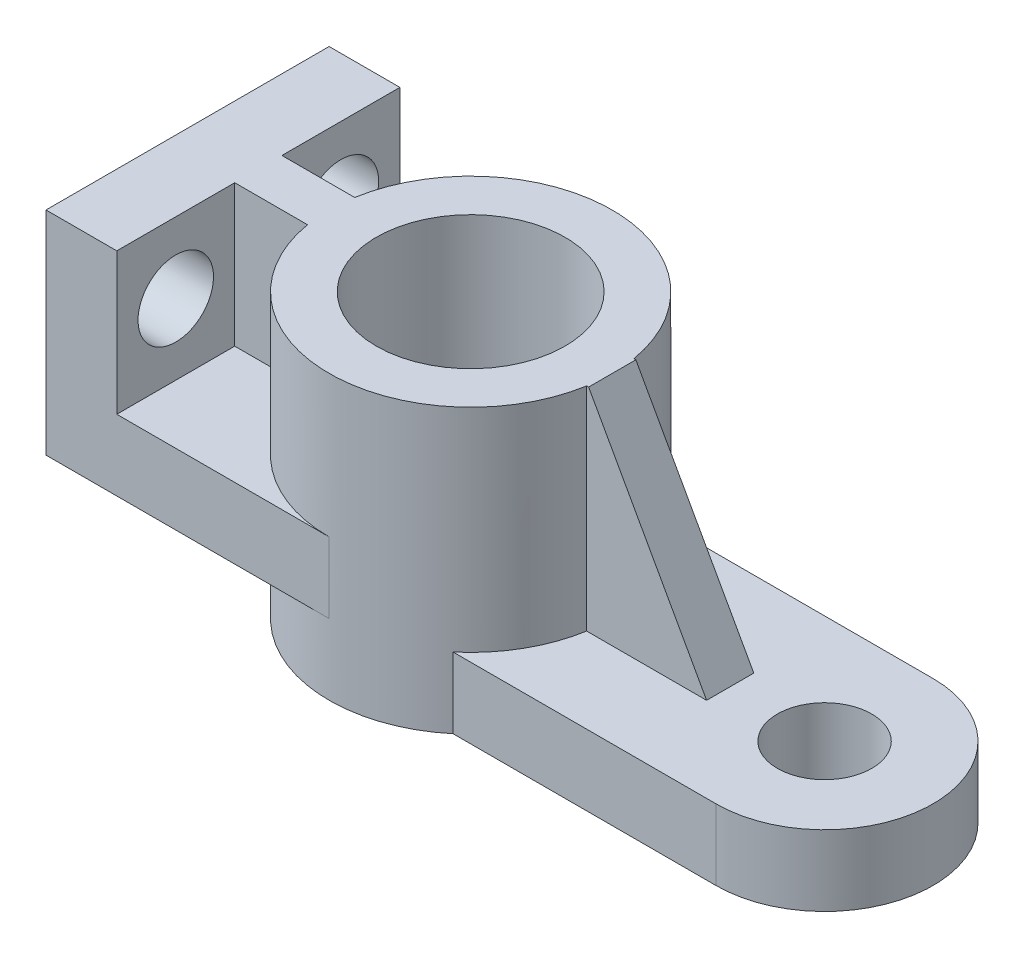
ISO-10303-21;
HEADER;
FILE_DESCRIPTION(('STEP AP214'),'2;1');
FILE_NAME('part.step','',(''),(''),'','','');
FILE_SCHEMA(('AUTOMOTIVE_DESIGN { 1 0 10303 214 1 1 1 1 }'));
ENDSEC;
DATA;
#1=APPLICATION_CONTEXT('core data for automotive mechanical design processes');
#2=APPLICATION_PROTOCOL_DEFINITION('international standard','automotive_design',2000,#1);
#3=PRODUCT_CONTEXT('',#1,'mechanical');
#4=PRODUCT('Part','Part','',(#3));
#5=PRODUCT_RELATED_PRODUCT_CATEGORY('part','',(#4));
#6=PRODUCT_DEFINITION_FORMATION('','',#4);
#7=PRODUCT_DEFINITION_CONTEXT('part definition',#1,'design');
#8=PRODUCT_DEFINITION('design','',#6,#7);
#9=PRODUCT_DEFINITION_SHAPE('','',#8);
#10=(LENGTH_UNIT() NAMED_UNIT(*) SI_UNIT(.MILLI.,.METRE.));
#11=(NAMED_UNIT(*) PLANE_ANGLE_UNIT() SI_UNIT($,.RADIAN.));
#12=(NAMED_UNIT(*) SI_UNIT($,.STERADIAN.) SOLID_ANGLE_UNIT());
#13=UNCERTAINTY_MEASURE_WITH_UNIT(LENGTH_MEASURE(1.E-05),#10,'distance_accuracy_value','');
#14=(GEOMETRIC_REPRESENTATION_CONTEXT(3) GLOBAL_UNCERTAINTY_ASSIGNED_CONTEXT((#13)) GLOBAL_UNIT_ASSIGNED_CONTEXT((#10,
#11,#12)) REPRESENTATION_CONTEXT('',''));
#15=CARTESIAN_POINT('',(0.,0.,0.));
#16=DIRECTION('',(0.,0.,1.));
#17=DIRECTION('',(1.,0.,0.));
#18=AXIS2_PLACEMENT_3D('',#15,#16,#17);
#19=CARTESIAN_POINT('',(0.,60.,0.));
#20=DIRECTION('',(0.,-1.,0.));
#21=DIRECTION('',(0.,0.,-1.));
#22=AXIS2_PLACEMENT_3D('',#19,#20,#21);
#23=CYLINDRICAL_SURFACE('',#22,30.);
#24=CARTESIAN_POINT('',(0.,15.,0.));
#25=DIRECTION('',(0.,-1.,0.));
#26=DIRECTION('',(0.,0.,-1.));
#27=AXIS2_PLACEMENT_3D('',#24,#25,#26);
#28=CIRCLE('',#27,30.);
#29=CARTESIAN_POINT('',(29.5803989154981,15.,5.));
#30=VERTEX_POINT('',#29);
#31=CARTESIAN_POINT('',(19.2613602842582,15.,23.));
#32=VERTEX_POINT('',#31);
#33=EDGE_CURVE('E251',#30,#32,#28,.T.);
#34=ORIENTED_EDGE('',*,*,#33,.F.);
#35=DIRECTION('',(0.,-1.,0.));
#36=VECTOR('',#35,1.);
#37=CARTESIAN_POINT('',(29.5803989154981,60.,5.));
#38=LINE('',#37,#36);
#39=CARTESIAN_POINT('',(29.5803989154981,60.,5.));
#40=VERTEX_POINT('',#39);
#41=EDGE_CURVE('E64',#30,#40,#38,.F.);
#42=ORIENTED_EDGE('',*,*,#41,.T.);
#43=CARTESIAN_POINT('',(0.,60.,0.));
#44=DIRECTION('',(0.,1.,0.));
#45=DIRECTION('',(0.,0.,1.));
#46=AXIS2_PLACEMENT_3D('',#43,#44,#45);
#47=CIRCLE('',#46,30.);
#48=CARTESIAN_POINT('',(-29.5803989154981,60.,5.));
#49=VERTEX_POINT('',#48);
#50=EDGE_CURVE('E189',#49,#40,#47,.T.);
#51=ORIENTED_EDGE('',*,*,#50,.F.);
#52=DIRECTION('',(0.,-1.,0.));
#53=VECTOR('',#52,1.);
#54=CARTESIAN_POINT('',(-29.5803989154981,60.,5.));
#55=LINE('',#54,#53);
#56=CARTESIAN_POINT('',(-29.5803989154981,30.,5.));
#57=VERTEX_POINT('',#56);
#58=EDGE_CURVE('E211',#57,#49,#55,.F.);
#59=ORIENTED_EDGE('',*,*,#58,.F.);
#60=CARTESIAN_POINT('',(0.,30.,0.));
#61=DIRECTION('',(0.,1.,0.));
#62=DIRECTION('',(0.,0.,1.));
#63=AXIS2_PLACEMENT_3D('',#60,#61,#62);
#64=CIRCLE('',#63,30.);
#65=CARTESIAN_POINT('',(0.,30.,30.));
#66=VERTEX_POINT('',#65);
#67=EDGE_CURVE('E268',#66,#57,#64,.F.);
#68=ORIENTED_EDGE('',*,*,#67,.F.);
#69=DIRECTION('',(0.,-1.,0.));
#70=VECTOR('',#69,1.);
#71=CARTESIAN_POINT('',(0.,0.,30.));
#72=LINE('',#71,#70);
#73=CARTESIAN_POINT('',(0.,15.,30.));
#74=VERTEX_POINT('',#73);
#75=EDGE_CURVE('E282',#66,#74,#72,.T.);
#76=ORIENTED_EDGE('',*,*,#75,.T.);
#77=CARTESIAN_POINT('',(0.,15.,0.));
#78=DIRECTION('',(0.,1.,0.));
#79=DIRECTION('',(-1.,0.,0.));
#80=AXIS2_PLACEMENT_3D('',#77,#78,#79);
#81=CIRCLE('',#80,30.);
#82=CARTESIAN_POINT('',(0.,15.,-30.));
#83=VERTEX_POINT('',#82);
#84=EDGE_CURVE('E275',#74,#83,#81,.F.);
#85=ORIENTED_EDGE('',*,*,#84,.T.);
#86=DIRECTION('',(0.,-1.,0.));
#87=VECTOR('',#86,1.);
#88=CARTESIAN_POINT('',(0.,0.,-30.));
#89=LINE('',#88,#87);
#90=CARTESIAN_POINT('',(0.,30.,-30.));
#91=VERTEX_POINT('',#90);
#92=EDGE_CURVE('E299',#91,#83,#89,.T.);
#93=ORIENTED_EDGE('',*,*,#92,.F.);
#94=CARTESIAN_POINT('',(-29.5803989154981,30.,-5.));
#95=VERTEX_POINT('',#94);
#96=EDGE_CURVE('E270',#95,#91,#64,.F.);
#97=ORIENTED_EDGE('',*,*,#96,.F.);
#98=DIRECTION('',(0.,-1.,0.));
#99=VECTOR('',#98,1.);
#100=CARTESIAN_POINT('',(-29.5803989154981,60.,-5.));
#101=LINE('',#100,#99);
#102=CARTESIAN_POINT('',(-29.5803989154981,60.,-5.));
#103=VERTEX_POINT('',#102);
#104=EDGE_CURVE('E215',#103,#95,#101,.T.);
#105=ORIENTED_EDGE('',*,*,#104,.F.);
#106=CARTESIAN_POINT('',(29.5803989154981,60.,-5.));
#107=VERTEX_POINT('',#106);
#108=EDGE_CURVE('E57',#107,#103,#47,.T.);
#109=ORIENTED_EDGE('',*,*,#108,.F.);
#110=DIRECTION('',(0.,-1.,0.));
#111=VECTOR('',#110,1.);
#112=CARTESIAN_POINT('',(29.5803989154981,60.,-5.));
#113=LINE('',#112,#111);
#114=CARTESIAN_POINT('',(29.5803989154981,15.,-5.));
#115=VERTEX_POINT('',#114);
#116=EDGE_CURVE('E193',#115,#107,#113,.F.);
#117=ORIENTED_EDGE('',*,*,#116,.F.);
#118=CARTESIAN_POINT('',(19.2613602842582,15.,-23.));
#119=VERTEX_POINT('',#118);
#120=EDGE_CURVE('E260',#119,#115,#28,.T.);
#121=ORIENTED_EDGE('',*,*,#120,.F.);
#122=DIRECTION('',(0.,1.,0.));
#123=VECTOR('',#122,1.);
#124=CARTESIAN_POINT('',(19.2613602842582,0.,-23.));
#125=LINE('',#124,#123);
#126=CARTESIAN_POINT('',(19.2613602842582,0.,-23.));
#127=VERTEX_POINT('',#126);
#128=EDGE_CURVE('E235',#127,#119,#125,.T.);
#129=ORIENTED_EDGE('',*,*,#128,.F.);
#130=CARTESIAN_POINT('',(0.,0.,0.));
#131=DIRECTION('',(0.,1.,0.));
#132=DIRECTION('',(0.,0.,1.));
#133=AXIS2_PLACEMENT_3D('',#130,#131,#132);
#134=CIRCLE('',#133,30.);
#135=CARTESIAN_POINT('',(19.2613602842582,0.,23.));
#136=VERTEX_POINT('',#135);
#137=EDGE_CURVE('E264',#127,#136,#134,.T.);
#138=ORIENTED_EDGE('',*,*,#137,.T.);
#139=DIRECTION('',(0.,1.,0.));
#140=VECTOR('',#139,1.);
#141=CARTESIAN_POINT('',(19.2613602842582,0.,23.));
#142=LINE('',#141,#140);
#143=EDGE_CURVE('E232',#136,#32,#142,.T.);
#144=ORIENTED_EDGE('',*,*,#143,.T.);
#145=EDGE_LOOP('',(#34,#42,#51,#59,#68,#76,#85,#93,#97,#105,#109,#117,#121,#129,#138,#144));
#146=FACE_BOUND('',#145,.T.);
#147=ADVANCED_FACE('F41',(#146),#23,.T.);
#148=CARTESIAN_POINT('',(0.,30.,30.));
#149=DIRECTION('',(0.,1.,0.));
#150=DIRECTION('',(0.,0.,1.));
#151=AXIS2_PLACEMENT_3D('',#148,#149,#150);
#152=PLANE('',#151);
#153=ORIENTED_EDGE('',*,*,#67,.T.);
#154=DIRECTION('',(-1.,0.,0.));
#155=VECTOR('',#154,1.);
#156=CARTESIAN_POINT('',(-27.,30.,5.));
#157=LINE('',#156,#155);
#158=CARTESIAN_POINT('',(-45.,30.,5.));
#159=VERTEX_POINT('',#158);
#160=EDGE_CURVE('E210',#57,#159,#157,.T.);
#161=ORIENTED_EDGE('',*,*,#160,.T.);
#162=DIRECTION('',(0.,0.,-1.));
#163=VECTOR('',#162,1.);
#164=CARTESIAN_POINT('',(-45.,30.,30.));
#165=LINE('',#164,#163);
#166=CARTESIAN_POINT('',(-45.,30.,30.));
#167=VERTEX_POINT('',#166);
#168=EDGE_CURVE('E317',#167,#159,#165,.T.);
#169=ORIENTED_EDGE('',*,*,#168,.F.);
#170=DIRECTION('',(1.,0.,0.));
#171=VECTOR('',#170,1.);
#172=CARTESIAN_POINT('',(0.,30.,30.));
#173=LINE('',#172,#171);
#174=EDGE_CURVE('E283',#167,#66,#173,.T.);
#175=ORIENTED_EDGE('',*,*,#174,.T.);
#176=EDGE_LOOP('',(#153,#161,#169,#175));
#177=FACE_BOUND('',#176,.T.);
#178=ADVANCED_FACE('F334',(#177),#152,.T.);
#179=CARTESIAN_POINT('',(-45.,30.,-5.));
#180=VERTEX_POINT('',#179);
#181=CARTESIAN_POINT('',(-45.,30.,-30.));
#182=VERTEX_POINT('',#181);
#183=EDGE_CURVE('E314',#180,#182,#165,.T.);
#184=ORIENTED_EDGE('',*,*,#183,.F.);
#185=DIRECTION('',(-1.,0.,0.));
#186=VECTOR('',#185,1.);
#187=CARTESIAN_POINT('',(-27.,30.,-5.));
#188=LINE('',#187,#186);
#189=EDGE_CURVE('E204',#95,#180,#188,.T.);
#190=ORIENTED_EDGE('',*,*,#189,.F.);
#191=ORIENTED_EDGE('',*,*,#96,.T.);
#192=DIRECTION('',(1.,0.,0.));
#193=VECTOR('',#192,1.);
#194=CARTESIAN_POINT('',(0.,30.,-30.));
#195=LINE('',#194,#193);
#196=EDGE_CURVE('E305',#182,#91,#195,.T.);
#197=ORIENTED_EDGE('',*,*,#196,.F.);
#198=EDGE_LOOP('',(#184,#190,#191,#197));
#199=FACE_BOUND('',#198,.T.);
#200=ADVANCED_FACE('F345',(#199),#152,.T.);
#201=CARTESIAN_POINT('',(-45.,0.,30.));
#202=DIRECTION('',(1.,0.,0.));
#203=DIRECTION('',(0.,1.,0.));
#204=AXIS2_PLACEMENT_3D('',#201,#202,#203);
#205=PLANE('',#204);
#206=CARTESIAN_POINT('',(-45.,45.,17.5));
#207=DIRECTION('',(1.,0.,0.));
#208=DIRECTION('',(0.,1.,0.));
#209=AXIS2_PLACEMENT_3D('',#206,#207,#208);
#210=CIRCLE('',#209,8.);
#211=CARTESIAN_POINT('',(-45.,53.,17.5));
#212=VERTEX_POINT('',#211);
#213=EDGE_CURVE('E221',#212,#212,#210,.T.);
#214=ORIENTED_EDGE('',*,*,#213,.F.);
#215=EDGE_LOOP('',(#214));
#216=FACE_BOUND('',#215,.T.);
#217=ORIENTED_EDGE('',*,*,#168,.T.);
#218=DIRECTION('',(0.,-1.,0.));
#219=VECTOR('',#218,1.);
#220=CARTESIAN_POINT('',(-45.,30.,5.));
#221=LINE('',#220,#219);
#222=CARTESIAN_POINT('',(-45.,60.,5.));
#223=VERTEX_POINT('',#222);
#224=EDGE_CURVE('E199',#223,#159,#221,.T.);
#225=ORIENTED_EDGE('',*,*,#224,.F.);
#226=DIRECTION('',(0.,0.,-1.));
#227=VECTOR('',#226,1.);
#228=CARTESIAN_POINT('',(-45.,60.,30.));
#229=LINE('',#228,#227);
#230=CARTESIAN_POINT('',(-45.,60.,30.));
#231=VERTEX_POINT('',#230);
#232=EDGE_CURVE('E315',#231,#223,#229,.T.);
#233=ORIENTED_EDGE('',*,*,#232,.F.);
#234=DIRECTION('',(0.,-1.,0.));
#235=VECTOR('',#234,1.);
#236=CARTESIAN_POINT('',(-45.,0.,30.));
#237=LINE('',#236,#235);
#238=EDGE_CURVE('E290',#231,#167,#237,.T.);
#239=ORIENTED_EDGE('',*,*,#238,.T.);
#240=EDGE_LOOP('',(#217,#225,#233,#239));
#241=FACE_BOUND('',#240,.T.);
#242=ADVANCED_FACE('F361',(#216,#241),#205,.T.);
#243=CARTESIAN_POINT('',(-45.,45.,-17.5));
#244=DIRECTION('',(1.,0.,0.));
#245=DIRECTION('',(0.,-1.,0.));
#246=AXIS2_PLACEMENT_3D('',#243,#244,#245);
#247=CIRCLE('',#246,8.);
#248=CARTESIAN_POINT('',(-45.,37.,-17.5));
#249=VERTEX_POINT('',#248);
#250=EDGE_CURVE('E216',#249,#249,#247,.T.);
#251=ORIENTED_EDGE('',*,*,#250,.F.);
#252=EDGE_LOOP('',(#251));
#253=FACE_BOUND('',#252,.T.);
#254=CARTESIAN_POINT('',(-45.,60.,-5.));
#255=VERTEX_POINT('',#254);
#256=CARTESIAN_POINT('',(-45.,60.,-30.));
#257=VERTEX_POINT('',#256);
#258=EDGE_CURVE('E311',#255,#257,#229,.T.);
#259=ORIENTED_EDGE('',*,*,#258,.F.);
#260=DIRECTION('',(0.,1.,0.));
#261=VECTOR('',#260,1.);
#262=CARTESIAN_POINT('',(-45.,60.,-5.));
#263=LINE('',#262,#261);
#264=EDGE_CURVE('E200',#180,#255,#263,.T.);
#265=ORIENTED_EDGE('',*,*,#264,.F.);
#266=ORIENTED_EDGE('',*,*,#183,.T.);
#267=DIRECTION('',(0.,-1.,0.));
#268=VECTOR('',#267,1.);
#269=CARTESIAN_POINT('',(-45.,0.,-30.));
#270=LINE('',#269,#268);
#271=EDGE_CURVE('E304',#257,#182,#270,.T.);
#272=ORIENTED_EDGE('',*,*,#271,.F.);
#273=EDGE_LOOP('',(#259,#265,#266,#272));
#274=FACE_BOUND('',#273,.T.);
#275=ADVANCED_FACE('F362',(#253,#274),#205,.T.);
#276=CARTESIAN_POINT('',(0.,15.,30.));
#277=DIRECTION('',(0.,1.,0.));
#278=DIRECTION('',(-1.,0.,0.));
#279=AXIS2_PLACEMENT_3D('',#276,#277,#278);
#280=PLANE('',#279);
#281=ORIENTED_EDGE('',*,*,#84,.F.);
#282=DIRECTION('',(1.,0.,0.));
#283=VECTOR('',#282,1.);
#284=CARTESIAN_POINT('',(0.,15.,30.));
#285=LINE('',#284,#283);
#286=CARTESIAN_POINT('',(-60.,15.,30.));
#287=VERTEX_POINT('',#286);
#288=EDGE_CURVE('E279',#287,#74,#285,.T.);
#289=ORIENTED_EDGE('',*,*,#288,.F.);
#290=DIRECTION('',(0.,0.,-1.));
#291=VECTOR('',#290,1.);
#292=CARTESIAN_POINT('',(-60.,15.,30.));
#293=LINE('',#292,#291);
#294=CARTESIAN_POINT('',(-60.,15.,-30.));
#295=VERTEX_POINT('',#294);
#296=EDGE_CURVE('E316',#287,#295,#293,.T.);
#297=ORIENTED_EDGE('',*,*,#296,.T.);
#298=DIRECTION('',(1.,0.,0.));
#299=VECTOR('',#298,1.);
#300=CARTESIAN_POINT('',(0.,15.,-30.));
#301=LINE('',#300,#299);
#302=EDGE_CURVE('E298',#295,#83,#301,.T.);
#303=ORIENTED_EDGE('',*,*,#302,.T.);
#304=EDGE_LOOP('',(#281,#289,#297,#303));
#305=FACE_BOUND('',#304,.T.);
#306=ADVANCED_FACE('F370',(#305),#280,.F.);
#307=CARTESIAN_POINT('',(-60.,0.,30.));
#308=DIRECTION('',(-1.,0.,0.));
#309=DIRECTION('',(0.,0.,1.));
#310=AXIS2_PLACEMENT_3D('',#307,#308,#309);
#311=PLANE('',#310);
#312=CARTESIAN_POINT('',(-60.,45.,17.5));
#313=DIRECTION('',(1.,0.,0.));
#314=DIRECTION('',(0.,1.,0.));
#315=AXIS2_PLACEMENT_3D('',#312,#313,#314);
#316=CIRCLE('',#315,8.);
#317=CARTESIAN_POINT('',(-60.,53.,17.5));
#318=VERTEX_POINT('',#317);
#319=EDGE_CURVE('E217',#318,#318,#316,.T.);
#320=ORIENTED_EDGE('',*,*,#319,.T.);
#321=EDGE_LOOP('',(#320));
#322=FACE_BOUND('',#321,.T.);
#323=CARTESIAN_POINT('',(-60.,45.,-17.5));
#324=DIRECTION('',(1.,0.,0.));
#325=DIRECTION('',(0.,-1.,0.));
#326=AXIS2_PLACEMENT_3D('',#323,#324,#325);
#327=CIRCLE('',#326,8.);
#328=CARTESIAN_POINT('',(-60.,37.,-17.5));
#329=VERTEX_POINT('',#328);
#330=EDGE_CURVE('E223',#329,#329,#327,.T.);
#331=ORIENTED_EDGE('',*,*,#330,.T.);
#332=EDGE_LOOP('',(#331));
#333=FACE_BOUND('',#332,.T.);
#334=DIRECTION('',(0.,1.,0.));
#335=VECTOR('',#334,1.);
#336=CARTESIAN_POINT('',(-60.,0.,-30.));
#337=LINE('',#336,#335);
#338=CARTESIAN_POINT('',(-60.,60.,-30.));
#339=VERTEX_POINT('',#338);
#340=EDGE_CURVE('E274',#295,#339,#337,.T.);
#341=ORIENTED_EDGE('',*,*,#340,.F.);
#342=ORIENTED_EDGE('',*,*,#296,.F.);
#343=DIRECTION('',(0.,1.,0.));
#344=VECTOR('',#343,1.);
#345=CARTESIAN_POINT('',(-60.,0.,30.));
#346=LINE('',#345,#344);
#347=CARTESIAN_POINT('',(-60.,60.,30.));
#348=VERTEX_POINT('',#347);
#349=EDGE_CURVE('E273',#287,#348,#346,.T.);
#350=ORIENTED_EDGE('',*,*,#349,.T.);
#351=DIRECTION('',(0.,0.,-1.));
#352=VECTOR('',#351,1.);
#353=CARTESIAN_POINT('',(-60.,60.,30.));
#354=LINE('',#353,#352);
#355=EDGE_CURVE('E291',#348,#339,#354,.T.);
#356=ORIENTED_EDGE('',*,*,#355,.T.);
#357=EDGE_LOOP('',(#341,#342,#350,#356));
#358=FACE_BOUND('',#357,.T.);
#359=ADVANCED_FACE('F43',(#322,#333,#358),#311,.T.);
#360=CARTESIAN_POINT('',(0.,60.,30.));
#361=DIRECTION('',(0.,1.,0.));
#362=DIRECTION('',(0.,0.,1.));
#363=AXIS2_PLACEMENT_3D('',#360,#361,#362);
#364=PLANE('',#363);
#365=CARTESIAN_POINT('',(0.,60.,0.));
#366=DIRECTION('',(0.,1.,0.));
#367=DIRECTION('',(0.,0.,1.));
#368=AXIS2_PLACEMENT_3D('',#365,#366,#367);
#369=CIRCLE('',#368,20.);
#370=CARTESIAN_POINT('',(0.,60.,20.));
#371=VERTEX_POINT('',#370);
#372=EDGE_CURVE('E258',#371,#371,#369,.T.);
#373=ORIENTED_EDGE('',*,*,#372,.F.);
#374=EDGE_LOOP('',(#373));
#375=FACE_BOUND('',#374,.T.);
#376=ORIENTED_EDGE('',*,*,#50,.T.);
#377=DIRECTION('',(-1.,0.,0.));
#378=VECTOR('',#377,1.);
#379=CARTESIAN_POINT('',(30.,60.,5.));
#380=LINE('',#379,#378);
#381=CARTESIAN_POINT('',(30.,60.,5.));
#382=VERTEX_POINT('',#381);
#383=EDGE_CURVE('E183',#382,#40,#380,.T.);
#384=ORIENTED_EDGE('',*,*,#383,.F.);
#385=DIRECTION('',(0.,0.,-1.));
#386=VECTOR('',#385,1.);
#387=CARTESIAN_POINT('',(30.,60.,5.));
#388=LINE('',#387,#386);
#389=CARTESIAN_POINT('',(30.,60.,-5.));
#390=VERTEX_POINT('',#389);
#391=EDGE_CURVE('E170',#382,#390,#388,.T.);
#392=ORIENTED_EDGE('',*,*,#391,.T.);
#393=DIRECTION('',(-1.,0.,0.));
#394=VECTOR('',#393,1.);
#395=CARTESIAN_POINT('',(30.,60.,-5.));
#396=LINE('',#395,#394);
#397=EDGE_CURVE('E188',#390,#107,#396,.T.);
#398=ORIENTED_EDGE('',*,*,#397,.T.);
#399=ORIENTED_EDGE('',*,*,#108,.T.);
#400=DIRECTION('',(-1.,0.,0.));
#401=VECTOR('',#400,1.);
#402=CARTESIAN_POINT('',(-27.,60.,-5.));
#403=LINE('',#402,#401);
#404=EDGE_CURVE('E205',#103,#255,#403,.T.);
#405=ORIENTED_EDGE('',*,*,#404,.T.);
#406=ORIENTED_EDGE('',*,*,#258,.T.);
#407=DIRECTION('',(1.,0.,0.));
#408=VECTOR('',#407,1.);
#409=CARTESIAN_POINT('',(0.,60.,-30.));
#410=LINE('',#409,#408);
#411=EDGE_CURVE('E276',#339,#257,#410,.T.);
#412=ORIENTED_EDGE('',*,*,#411,.F.);
#413=ORIENTED_EDGE('',*,*,#355,.F.);
#414=DIRECTION('',(1.,0.,0.));
#415=VECTOR('',#414,1.);
#416=CARTESIAN_POINT('',(0.,60.,30.));
#417=LINE('',#416,#415);
#418=EDGE_CURVE('E289',#348,#231,#417,.T.);
#419=ORIENTED_EDGE('',*,*,#418,.T.);
#420=ORIENTED_EDGE('',*,*,#232,.T.);
#421=DIRECTION('',(-1.,0.,0.));
#422=VECTOR('',#421,1.);
#423=CARTESIAN_POINT('',(-27.,60.,5.));
#424=LINE('',#423,#422);
#425=EDGE_CURVE('E208',#49,#223,#424,.T.);
#426=ORIENTED_EDGE('',*,*,#425,.F.);
#427=EDGE_LOOP('',(#376,#384,#392,#398,#399,#405,#406,#412,#413,#419,#420,#426));
#428=FACE_BOUND('',#427,.T.);
#429=ADVANCED_FACE('F187',(#375,#428),#364,.T.);
#430=CARTESIAN_POINT('',(0.,0.,30.));
#431=DIRECTION('',(0.,0.,1.));
#432=DIRECTION('',(1.,0.,0.));
#433=AXIS2_PLACEMENT_3D('',#430,#431,#432);
#434=PLANE('',#433);
#435=ORIENTED_EDGE('',*,*,#349,.F.);
#436=ORIENTED_EDGE('',*,*,#288,.T.);
#437=ORIENTED_EDGE('',*,*,#75,.F.);
#438=ORIENTED_EDGE('',*,*,#174,.F.);
#439=ORIENTED_EDGE('',*,*,#238,.F.);
#440=ORIENTED_EDGE('',*,*,#418,.F.);
#441=EDGE_LOOP('',(#435,#436,#437,#438,#439,#440));
#442=FACE_BOUND('',#441,.T.);
#443=ADVANCED_FACE('F352',(#442),#434,.T.);
#444=CARTESIAN_POINT('',(0.,0.,-30.));
#445=DIRECTION('',(0.,0.,1.));
#446=DIRECTION('',(1.,0.,0.));
#447=AXIS2_PLACEMENT_3D('',#444,#445,#446);
#448=PLANE('',#447);
#449=ORIENTED_EDGE('',*,*,#340,.T.);
#450=ORIENTED_EDGE('',*,*,#411,.T.);
#451=ORIENTED_EDGE('',*,*,#271,.T.);
#452=ORIENTED_EDGE('',*,*,#196,.T.);
#453=ORIENTED_EDGE('',*,*,#92,.T.);
#454=ORIENTED_EDGE('',*,*,#302,.F.);
#455=EDGE_LOOP('',(#449,#450,#451,#452,#453,#454));
#456=FACE_BOUND('',#455,.T.);
#457=ADVANCED_FACE('F358',(#456),#448,.F.);
#458=CARTESIAN_POINT('',(0.,0.,0.));
#459=DIRECTION('',(0.,1.,0.));
#460=DIRECTION('',(0.,0.,1.));
#461=AXIS2_PLACEMENT_3D('',#458,#459,#460);
#462=PLANE('',#461);
#463=CARTESIAN_POINT('',(75.,0.,0.));
#464=DIRECTION('',(0.,1.,0.));
#465=DIRECTION('',(0.,0.,1.));
#466=AXIS2_PLACEMENT_3D('',#463,#464,#465);
#467=CIRCLE('',#466,9.99999999999999);
#468=CARTESIAN_POINT('',(75.,0.,9.99999999999999));
#469=VERTEX_POINT('',#468);
#470=EDGE_CURVE('E244',#469,#469,#467,.T.);
#471=ORIENTED_EDGE('',*,*,#470,.T.);
#472=EDGE_LOOP('',(#471));
#473=FACE_BOUND('',#472,.T.);
#474=CARTESIAN_POINT('',(75.,0.,0.));
#475=DIRECTION('',(0.,1.,0.));
#476=DIRECTION('',(0.,0.,1.));
#477=AXIS2_PLACEMENT_3D('',#474,#475,#476);
#478=CIRCLE('',#477,23.);
#479=CARTESIAN_POINT('',(75.,0.,23.));
#480=VERTEX_POINT('',#479);
#481=CARTESIAN_POINT('',(75.,0.,-23.));
#482=VERTEX_POINT('',#481);
#483=EDGE_CURVE('E247',#480,#482,#478,.T.);
#484=ORIENTED_EDGE('',*,*,#483,.F.);
#485=DIRECTION('',(-1.,0.,0.));
#486=VECTOR('',#485,1.);
#487=CARTESIAN_POINT('',(74.9999999999999,0.,23.));
#488=LINE('',#487,#486);
#489=EDGE_CURVE('E238',#480,#136,#488,.T.);
#490=ORIENTED_EDGE('',*,*,#489,.T.);
#491=ORIENTED_EDGE('',*,*,#137,.F.);
#492=DIRECTION('',(1.,0.,0.));
#493=VECTOR('',#492,1.);
#494=CARTESIAN_POINT('',(75.,0.,-23.));
#495=LINE('',#494,#493);
#496=EDGE_CURVE('E230',#127,#482,#495,.T.);
#497=ORIENTED_EDGE('',*,*,#496,.T.);
#498=EDGE_LOOP('',(#484,#490,#491,#497));
#499=FACE_BOUND('',#498,.T.);
#500=CARTESIAN_POINT('',(0.,0.,0.));
#501=DIRECTION('',(0.,1.,0.));
#502=DIRECTION('',(0.,0.,1.));
#503=AXIS2_PLACEMENT_3D('',#500,#501,#502);
#504=CIRCLE('',#503,20.);
#505=CARTESIAN_POINT('',(0.,0.,20.));
#506=VERTEX_POINT('',#505);
#507=EDGE_CURVE('E256',#506,#506,#504,.T.);
#508=ORIENTED_EDGE('',*,*,#507,.T.);
#509=EDGE_LOOP('',(#508));
#510=FACE_BOUND('',#509,.T.);
#511=ADVANCED_FACE('F347',(#473,#499,#510),#462,.F.);
#512=CARTESIAN_POINT('',(0.,60.,0.));
#513=DIRECTION('',(0.,-1.,0.));
#514=DIRECTION('',(0.,0.,-1.));
#515=AXIS2_PLACEMENT_3D('',#512,#513,#514);
#516=CYLINDRICAL_SURFACE('',#515,20.);
#517=ORIENTED_EDGE('',*,*,#507,.F.);
#518=EDGE_LOOP('',(#517));
#519=FACE_BOUND('',#518,.T.);
#520=ORIENTED_EDGE('',*,*,#372,.T.);
#521=EDGE_LOOP('',(#520));
#522=FACE_BOUND('',#521,.T.);
#523=ADVANCED_FACE('F348',(#519,#522),#516,.F.);
#524=CARTESIAN_POINT('',(0.,15.,30.));
#525=DIRECTION('',(0.,-1.,0.));
#526=DIRECTION('',(0.,0.,-1.));
#527=AXIS2_PLACEMENT_3D('',#524,#525,#526);
#528=PLANE('',#527);
#529=CARTESIAN_POINT('',(75.,15.,0.));
#530=DIRECTION('',(0.,1.,0.));
#531=DIRECTION('',(0.,0.,1.));
#532=AXIS2_PLACEMENT_3D('',#529,#530,#531);
#533=CIRCLE('',#532,9.99999999999999);
#534=CARTESIAN_POINT('',(75.,15.,9.99999999999999));
#535=VERTEX_POINT('',#534);
#536=EDGE_CURVE('E240',#535,#535,#533,.T.);
#537=ORIENTED_EDGE('',*,*,#536,.F.);
#538=EDGE_LOOP('',(#537));
#539=FACE_BOUND('',#538,.T.);
#540=DIRECTION('',(0.,0.,-1.));
#541=VECTOR('',#540,1.);
#542=CARTESIAN_POINT('',(55.,15.,5.));
#543=LINE('',#542,#541);
#544=CARTESIAN_POINT('',(55.,15.,5.));
#545=VERTEX_POINT('',#544);
#546=CARTESIAN_POINT('',(55.,15.,-5.));
#547=VERTEX_POINT('',#546);
#548=EDGE_CURVE('E178',#545,#547,#543,.T.);
#549=ORIENTED_EDGE('',*,*,#548,.F.);
#550=DIRECTION('',(-1.,0.,0.));
#551=VECTOR('',#550,1.);
#552=CARTESIAN_POINT('',(0.,15.,5.));
#553=LINE('',#552,#551);
#554=EDGE_CURVE('E11',#545,#30,#553,.T.);
#555=ORIENTED_EDGE('',*,*,#554,.T.);
#556=ORIENTED_EDGE('',*,*,#33,.T.);
#557=DIRECTION('',(-1.,0.,0.));
#558=VECTOR('',#557,1.);
#559=CARTESIAN_POINT('',(74.9999999999999,15.,23.));
#560=LINE('',#559,#558);
#561=CARTESIAN_POINT('',(74.9999999999999,15.,23.));
#562=VERTEX_POINT('',#561);
#563=EDGE_CURVE('E220',#562,#32,#560,.T.);
#564=ORIENTED_EDGE('',*,*,#563,.F.);
#565=CARTESIAN_POINT('',(75.,15.,0.));
#566=DIRECTION('',(0.,1.,0.));
#567=DIRECTION('',(0.,0.,1.));
#568=AXIS2_PLACEMENT_3D('',#565,#566,#567);
#569=CIRCLE('',#568,23.);
#570=CARTESIAN_POINT('',(75.,15.,-23.));
#571=VERTEX_POINT('',#570);
#572=EDGE_CURVE('E252',#562,#571,#569,.T.);
#573=ORIENTED_EDGE('',*,*,#572,.T.);
#574=DIRECTION('',(1.,0.,0.));
#575=VECTOR('',#574,1.);
#576=CARTESIAN_POINT('',(75.,15.,-23.));
#577=LINE('',#576,#575);
#578=EDGE_CURVE('E231',#119,#571,#577,.T.);
#579=ORIENTED_EDGE('',*,*,#578,.F.);
#580=ORIENTED_EDGE('',*,*,#120,.T.);
#581=DIRECTION('',(-1.,0.,0.));
#582=VECTOR('',#581,1.);
#583=CARTESIAN_POINT('',(0.,15.,-5.));
#584=LINE('',#583,#582);
#585=EDGE_CURVE('E47',#547,#115,#584,.T.);
#586=ORIENTED_EDGE('',*,*,#585,.F.);
#587=EDGE_LOOP('',(#549,#555,#556,#564,#573,#579,#580,#586));
#588=FACE_BOUND('',#587,.T.);
#589=ADVANCED_FACE('F330',(#539,#588),#528,.F.);
#590=CARTESIAN_POINT('',(75.,15.,0.));
#591=DIRECTION('',(0.,-1.,0.));
#592=DIRECTION('',(0.,0.,-1.));
#593=AXIS2_PLACEMENT_3D('',#590,#591,#592);
#594=CYLINDRICAL_SURFACE('',#593,23.);
#595=ORIENTED_EDGE('',*,*,#483,.T.);
#596=DIRECTION('',(0.,-1.,0.));
#597=VECTOR('',#596,1.);
#598=CARTESIAN_POINT('',(75.,15.,-23.));
#599=LINE('',#598,#597);
#600=EDGE_CURVE('E321',#482,#571,#599,.F.);
#601=ORIENTED_EDGE('',*,*,#600,.T.);
#602=ORIENTED_EDGE('',*,*,#572,.F.);
#603=DIRECTION('',(0.,-1.,0.));
#604=VECTOR('',#603,1.);
#605=CARTESIAN_POINT('',(75.,15.,23.));
#606=LINE('',#605,#604);
#607=EDGE_CURVE('E322',#562,#480,#606,.T.);
#608=ORIENTED_EDGE('',*,*,#607,.T.);
#609=EDGE_LOOP('',(#595,#601,#602,#608));
#610=FACE_BOUND('',#609,.T.);
#611=ADVANCED_FACE('F424',(#610),#594,.T.);
#612=CARTESIAN_POINT('',(75.,0.,-23.));
#613=DIRECTION('',(0.,0.,1.));
#614=DIRECTION('',(1.,0.,0.));
#615=AXIS2_PLACEMENT_3D('',#612,#613,#614);
#616=PLANE('',#615);
#617=ORIENTED_EDGE('',*,*,#578,.T.);
#618=ORIENTED_EDGE('',*,*,#600,.F.);
#619=ORIENTED_EDGE('',*,*,#496,.F.);
#620=ORIENTED_EDGE('',*,*,#128,.T.);
#621=EDGE_LOOP('',(#617,#618,#619,#620));
#622=FACE_BOUND('',#621,.T.);
#623=ADVANCED_FACE('F423',(#622),#616,.F.);
#624=CARTESIAN_POINT('',(74.9999999999999,0.,23.));
#625=DIRECTION('',(0.,0.,-1.));
#626=DIRECTION('',(-1.,0.,0.));
#627=AXIS2_PLACEMENT_3D('',#624,#625,#626);
#628=PLANE('',#627);
#629=ORIENTED_EDGE('',*,*,#563,.T.);
#630=ORIENTED_EDGE('',*,*,#143,.F.);
#631=ORIENTED_EDGE('',*,*,#489,.F.);
#632=ORIENTED_EDGE('',*,*,#607,.F.);
#633=EDGE_LOOP('',(#629,#630,#631,#632));
#634=FACE_BOUND('',#633,.T.);
#635=ADVANCED_FACE('F425',(#634),#628,.F.);
#636=CARTESIAN_POINT('',(75.,0.,0.));
#637=DIRECTION('',(0.,1.,0.));
#638=DIRECTION('',(0.,0.,1.));
#639=AXIS2_PLACEMENT_3D('',#636,#637,#638);
#640=CYLINDRICAL_SURFACE('',#639,9.99999999999999);
#641=ORIENTED_EDGE('',*,*,#470,.F.);
#642=EDGE_LOOP('',(#641));
#643=FACE_BOUND('',#642,.T.);
#644=ORIENTED_EDGE('',*,*,#536,.T.);
#645=EDGE_LOOP('',(#644));
#646=FACE_BOUND('',#645,.T.);
#647=ADVANCED_FACE('F418',(#643,#646),#640,.F.);
#648=CARTESIAN_POINT('',(-60.,45.,-17.5));
#649=DIRECTION('',(1.,0.,0.));
#650=DIRECTION('',(0.,1.,0.));
#651=AXIS2_PLACEMENT_3D('',#648,#649,#650);
#652=CYLINDRICAL_SURFACE('',#651,8.);
#653=ORIENTED_EDGE('',*,*,#330,.F.);
#654=EDGE_LOOP('',(#653));
#655=FACE_BOUND('',#654,.T.);
#656=ORIENTED_EDGE('',*,*,#250,.T.);
#657=EDGE_LOOP('',(#656));
#658=FACE_BOUND('',#657,.T.);
#659=ADVANCED_FACE('F412',(#655,#658),#652,.F.);
#660=CARTESIAN_POINT('',(-60.,45.,17.5));
#661=DIRECTION('',(1.,0.,0.));
#662=DIRECTION('',(0.,1.,0.));
#663=AXIS2_PLACEMENT_3D('',#660,#661,#662);
#664=CYLINDRICAL_SURFACE('',#663,8.);
#665=ORIENTED_EDGE('',*,*,#319,.F.);
#666=EDGE_LOOP('',(#665));
#667=FACE_BOUND('',#666,.T.);
#668=ORIENTED_EDGE('',*,*,#213,.T.);
#669=EDGE_LOOP('',(#668));
#670=FACE_BOUND('',#669,.T.);
#671=ADVANCED_FACE('F407',(#667,#670),#664,.F.);
#672=CARTESIAN_POINT('',(-27.,30.,5.));
#673=DIRECTION('',(0.,0.,-1.));
#674=DIRECTION('',(-1.,0.,0.));
#675=AXIS2_PLACEMENT_3D('',#672,#673,#674);
#676=PLANE('',#675);
#677=ORIENTED_EDGE('',*,*,#160,.F.);
#678=ORIENTED_EDGE('',*,*,#58,.T.);
#679=ORIENTED_EDGE('',*,*,#425,.T.);
#680=ORIENTED_EDGE('',*,*,#224,.T.);
#681=EDGE_LOOP('',(#677,#678,#679,#680));
#682=FACE_BOUND('',#681,.T.);
#683=ADVANCED_FACE('F404',(#682),#676,.F.);
#684=CARTESIAN_POINT('',(-27.,60.,-5.));
#685=DIRECTION('',(0.,0.,1.));
#686=DIRECTION('',(0.,-1.,0.));
#687=AXIS2_PLACEMENT_3D('',#684,#685,#686);
#688=PLANE('',#687);
#689=ORIENTED_EDGE('',*,*,#404,.F.);
#690=ORIENTED_EDGE('',*,*,#104,.T.);
#691=ORIENTED_EDGE('',*,*,#189,.T.);
#692=ORIENTED_EDGE('',*,*,#264,.T.);
#693=EDGE_LOOP('',(#689,#690,#691,#692));
#694=FACE_BOUND('',#693,.T.);
#695=ADVANCED_FACE('F396',(#694),#688,.F.);
#696=CARTESIAN_POINT('',(0.,0.,5.));
#697=DIRECTION('',(0.,0.,1.));
#698=DIRECTION('',(1.,0.,0.));
#699=AXIS2_PLACEMENT_3D('',#696,#697,#698);
#700=PLANE('',#699);
#701=ORIENTED_EDGE('',*,*,#41,.F.);
#702=ORIENTED_EDGE('',*,*,#554,.F.);
#703=DIRECTION('',(-0.485642931178632,0.874157276121538,0.));
#704=VECTOR('',#703,1.);
#705=CARTESIAN_POINT('',(55.,15.,5.));
#706=LINE('',#705,#704);
#707=EDGE_CURVE('E171',#545,#382,#706,.T.);
#708=ORIENTED_EDGE('',*,*,#707,.T.);
#709=ORIENTED_EDGE('',*,*,#383,.T.);
#710=EDGE_LOOP('',(#701,#702,#708,#709));
#711=FACE_BOUND('',#710,.T.);
#712=ADVANCED_FACE('F182',(#711),#700,.T.);
#713=CARTESIAN_POINT('',(0.,0.,-5.));
#714=DIRECTION('',(0.,0.,1.));
#715=DIRECTION('',(1.,0.,0.));
#716=AXIS2_PLACEMENT_3D('',#713,#714,#715);
#717=PLANE('',#716);
#718=ORIENTED_EDGE('',*,*,#585,.T.);
#719=ORIENTED_EDGE('',*,*,#116,.T.);
#720=ORIENTED_EDGE('',*,*,#397,.F.);
#721=DIRECTION('',(-0.485642931178632,0.874157276121538,0.));
#722=VECTOR('',#721,1.);
#723=CARTESIAN_POINT('',(55.,15.,-5.));
#724=LINE('',#723,#722);
#725=EDGE_CURVE('E173',#547,#390,#724,.T.);
#726=ORIENTED_EDGE('',*,*,#725,.F.);
#727=EDGE_LOOP('',(#718,#719,#720,#726));
#728=FACE_BOUND('',#727,.T.);
#729=ADVANCED_FACE('F329',(#728),#717,.F.);
#730=CARTESIAN_POINT('',(55.,15.,5.));
#731=DIRECTION('',(-0.874157276121538,-0.485642931178632,0.));
#732=DIRECTION('',(0.485642931178632,-0.874157276121538,0.));
#733=AXIS2_PLACEMENT_3D('',#730,#731,#732);
#734=PLANE('',#733);
#735=ORIENTED_EDGE('',*,*,#725,.T.);
#736=ORIENTED_EDGE('',*,*,#391,.F.);
#737=ORIENTED_EDGE('',*,*,#707,.F.);
#738=ORIENTED_EDGE('',*,*,#548,.T.);
#739=EDGE_LOOP('',(#735,#736,#737,#738));
#740=FACE_BOUND('',#739,.T.);
#741=ADVANCED_FACE('F169',(#740),#734,.F.);
#742=CLOSED_SHELL('',(#147,#178,#200,#242,#275,#306,#359,#429,#443,#457,#511,#523,#589,#611,
#623,#635,#647,#659,#671,#683,#695,#712,#729,#741));
#743=MANIFOLD_SOLID_BREP('B2',#742);
#744=ADVANCED_BREP_SHAPE_REPRESENTATION('',(#18,#743),#14);
#745=SHAPE_DEFINITION_REPRESENTATION(#9,#744);
ENDSEC;
END-ISO-10303-21;
